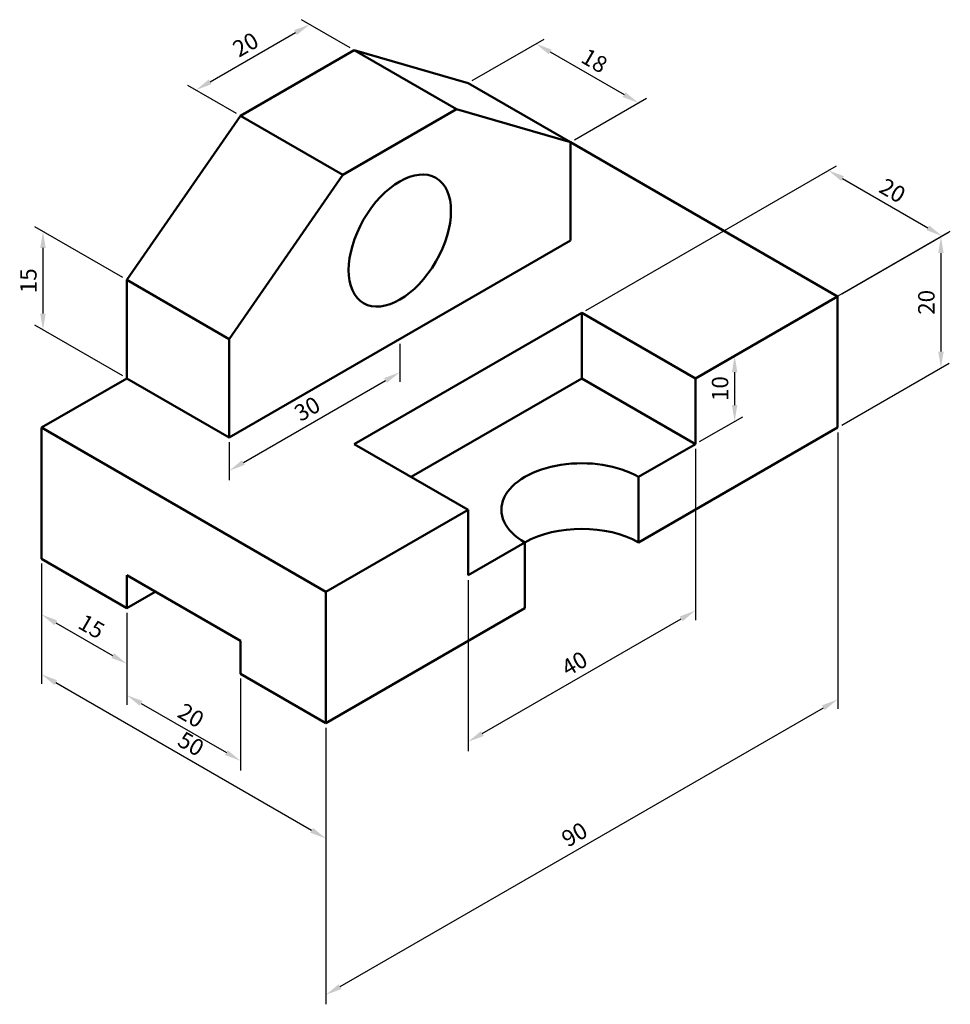
# Model space of a CAD drawing. Units: millimetres. Extents: x 3965 to 4107, y 1476 to 1626.
import ezdxf

# ---------------------------------------------------------------- set-up
doc = ezdxf.new("R2010")
doc.units = ezdxf.units.MM
doc.layers.add('M-DIMS', color=2, linetype='Continuous', lineweight=25)
doc.layers.add('M-OUTL', color=7, linetype='Continuous', lineweight=50)
doc.styles.get("Standard").update_dxf_attribs({"font": 'arial.ttf'})
doc.dimstyles.new('ISO-25', dxfattribs={"dimtxt": 2.5, "dimasz": 2.5, "dimexe": 1.25, "dimexo": 0.625, "dimtad": 1, "dimtxsty": 'Standard', "dimcen": 2.5, "dimadec": 0, "dimazin": 0, "dimtfac": 1, "dimtmove": 0, "dimatfit": 3, "dimfxl": 1, "dimarcsym": 0})

# ---------------------------------------------------------------- blocks, each defined once
blk = doc.blocks.new('*D1')
at = {"layer": 'Defpoints', "color": 0, "transparency": 16777216}
for p in [(3968.18, 1543.38), (4011.48, 1518.38), (4011.48, 1500.79)]:
    blk.add_point(p, dxfattribs=at)
at = {"layer": 'M-DIMS', "color": 0, "lineweight": -2, "transparency": 16777216}
for p, q in [((3968.18, 1542.66), (3968.18, 1524.34)), ((3970.35, 1524.54), (4009.32, 1502.04)), ((4011.48, 1517.66), (4011.48, 1499.34))]:
    blk.add_line(p, q, dxfattribs=at)
at = {"layer": 'M-DIMS', "color": 0, "transparency": 16777216}
for points in [[(3970.56, 1524.9), (3970.14, 1524.17), (3968.18, 1525.79)], [(4009.53, 1502.4), (4009.11, 1501.67), (4011.48, 1500.79)]]:
    blk.add_solid(points, dxfattribs=at)
at = {"layer": 'M-DIMS', "color": 0, "transparency": 16777216, "insert": (3990.78, 1514.93), "char_height": 2.5, "attachment_point": 5, "rotation": 330}
blk.add_mtext('50', dxfattribs=at)
blk = doc.blocks.new('*D2')
at = {"layer": 'Defpoints', "color": 0, "transparency": 16777216}
for p in [(3968.18, 1543.38), (3981.17, 1535.88), (3981.17, 1527.41)]:
    blk.add_point(p, dxfattribs=at)
at = {"layer": 'M-DIMS', "color": 0, "lineweight": -2, "transparency": 16777216}
for p, q in [((3968.18, 1542.66), (3968.18, 1533.47)), ((3981.17, 1535.16), (3981.17, 1525.97)), ((3970.35, 1533.66), (3979.01, 1528.66))]:
    blk.add_line(p, q, dxfattribs=at)
at = {"layer": 'M-DIMS', "color": 0, "transparency": 16777216}
for points in [[(3970.56, 1534.02), (3970.14, 1533.3), (3968.18, 1534.91)], [(3979.22, 1529.02), (3978.8, 1528.3), (3981.17, 1527.41)]]:
    blk.add_solid(points, dxfattribs=at)
at = {"layer": 'M-DIMS', "color": 0, "transparency": 16777216, "insert": (3975.63, 1532.81), "char_height": 2.5, "attachment_point": 5, "rotation": 330}
blk.add_mtext('15', dxfattribs=at)
blk = doc.blocks.new('*D3')
at = {"layer": 'Defpoints', "color": 0, "transparency": 16777216}
for p in [(3981.17, 1535.88), (3998.49, 1525.88), (3998.49, 1512.62)]:
    blk.add_point(p, dxfattribs=at)
at = {"layer": 'M-DIMS', "color": 0, "lineweight": -2, "transparency": 16777216}
for p, q in [((3981.17, 1535.16), (3981.17, 1521.17)), ((3998.49, 1525.16), (3998.49, 1511.17)), ((3983.34, 1521.37), (3996.33, 1513.87))]:
    blk.add_line(p, q, dxfattribs=at)
at = {"layer": 'M-DIMS', "color": 0, "transparency": 16777216}
for points in [[(3983.55, 1521.73), (3983.13, 1521.01), (3981.17, 1522.62)], [(3996.54, 1514.23), (3996.12, 1513.51), (3998.49, 1512.62)]]:
    blk.add_solid(points, dxfattribs=at)
at = {"layer": 'M-DIMS', "color": 0, "transparency": 16777216, "insert": (3990.78, 1519.26), "char_height": 2.5, "attachment_point": 5, "rotation": 330}
blk.add_mtext('20', dxfattribs=at)
blk = doc.blocks.new('*D4')
at = {"layer": 'Defpoints', "color": 0, "transparency": 16777216}
for p in [(4089.43, 1563.38), (4089.43, 1521.97), (4011.48, 1518.38)]:
    blk.add_point(p, dxfattribs=at)
at = {"layer": 'M-DIMS', "color": 0, "lineweight": -2, "transparency": 16777216}
for p, q in [((4089.43, 1562.66), (4089.43, 1520.53)), ((4013.65, 1478.22), (4087.26, 1520.72)), ((4011.48, 1517.66), (4011.48, 1475.53))]:
    blk.add_line(p, q, dxfattribs=at)
at = {"layer": 'M-DIMS', "color": 0, "transparency": 16777216}
for points in [[(4087.05, 1521.08), (4087.47, 1520.36), (4089.43, 1521.97)], [(4013.44, 1478.58), (4013.86, 1477.86), (4011.48, 1476.97)]]:
    blk.add_solid(points, dxfattribs=at)
at = {"layer": 'M-DIMS', "color": 0, "transparency": 16777216, "insert": (4049.5, 1501.12), "char_height": 2.5, "attachment_point": 5, "rotation": 30}
blk.add_mtext('90', dxfattribs=at)
blk = doc.blocks.new('*D5')
at = {"layer": 'Defpoints', "color": 0, "transparency": 16777216}
for p in [(4067.77, 1560.88), (4033.13, 1540.88), (4067.77, 1535.52)]:
    blk.add_point(p, dxfattribs=at)
at = {"layer": 'M-DIMS', "color": 0, "lineweight": -2, "transparency": 16777216}
for p, q in [((4067.77, 1560.16), (4067.77, 1534.07)), ((4033.13, 1540.16), (4033.13, 1514.07)), ((4035.3, 1516.77), (4065.61, 1534.27))]:
    blk.add_line(p, q, dxfattribs=at)
at = {"layer": 'M-DIMS', "color": 0, "transparency": 16777216}
for points in [[(4065.4, 1534.63), (4065.82, 1533.9), (4067.77, 1535.52)], [(4035.09, 1517.13), (4035.51, 1516.4), (4033.13, 1515.52)]]:
    blk.add_solid(points, dxfattribs=at)
at = {"layer": 'M-DIMS', "color": 0, "transparency": 16777216, "insert": (4049.5, 1527.16), "char_height": 2.5, "attachment_point": 5, "rotation": 30}
blk.add_mtext('40', dxfattribs=at)
blk = doc.blocks.new('*D6')
at = {"layer": 'Defpoints', "color": 0, "transparency": 16777216}
for p in [(4105.33, 1592.57), (4050.45, 1580.88), (4067.77, 1570.88)]:
    blk.add_point(p, dxfattribs=at)
at = {"layer": 'M-DIMS', "color": 0, "lineweight": -2, "transparency": 16777216}
for p, q in [((4051.08, 1581.25), (4089.26, 1603.29)), ((4090.18, 1601.32), (4103.17, 1593.82)), ((4068.4, 1571.25), (4106.58, 1593.29))]:
    blk.add_line(p, q, dxfattribs=at)
at = {"layer": 'M-DIMS', "color": 0, "transparency": 16777216}
for points in [[(4090.39, 1601.68), (4089.97, 1600.96), (4088.01, 1602.57)], [(4103.38, 1594.18), (4102.96, 1593.46), (4105.33, 1592.57)]]:
    blk.add_solid(points, dxfattribs=at)
at = {"layer": 'M-DIMS', "color": 0, "transparency": 16777216, "insert": (4097.62, 1599.22), "char_height": 2.5, "attachment_point": 5, "rotation": 330}
blk.add_mtext('20', dxfattribs=at)
blk = doc.blocks.new('*D7')
at = {"layer": 'Defpoints', "color": 0, "transparency": 16777216}
for p in [(4089.43, 1583.38), (4105.16, 1572.47), (4089.43, 1563.38)]:
    blk.add_point(p, dxfattribs=at)
at = {"layer": 'M-DIMS', "color": 0, "lineweight": -2, "transparency": 16777216}
for p, q in [((4090.05, 1583.75), (4106.41, 1593.19)), ((4105.16, 1589.97), (4105.16, 1574.97)), ((4090.05, 1563.75), (4106.41, 1573.19))]:
    blk.add_line(p, q, dxfattribs=at)
at = {"layer": 'M-DIMS', "color": 0, "transparency": 16777216}
for points in [[(4104.74, 1589.97), (4105.58, 1589.97), (4105.16, 1592.47)], [(4104.74, 1574.97), (4105.58, 1574.97), (4105.16, 1572.47)]]:
    blk.add_solid(points, dxfattribs=at)
at = {"layer": 'M-DIMS', "color": 0, "transparency": 16777216, "insert": (4103.26, 1582.47), "char_height": 2.5, "attachment_point": 5, "rotation": 90}
blk.add_mtext('20', dxfattribs=at)
blk = doc.blocks.new('*D8')
at = {"layer": 'Defpoints', "color": 0, "transparency": 16777216}
for p in [(4067.77, 1570.88), (4073.74, 1564.33), (4067.77, 1560.88)]:
    blk.add_point(p, dxfattribs=at)
at = {"layer": 'M-DIMS', "color": 0, "lineweight": -2, "transparency": 16777216}
for p, q in [((4068.4, 1571.25), (4074.99, 1575.05)), ((4073.74, 1571.83), (4073.74, 1566.83)), ((4068.4, 1561.25), (4074.99, 1565.05))]:
    blk.add_line(p, q, dxfattribs=at)
at = {"layer": 'M-DIMS', "color": 0, "transparency": 16777216}
for points in [[(4073.32, 1571.83), (4074.15, 1571.83), (4073.74, 1574.33)], [(4073.32, 1566.83), (4074.15, 1566.83), (4073.74, 1564.33)]]:
    blk.add_solid(points, dxfattribs=at)
at = {"layer": 'M-DIMS', "color": 0, "transparency": 16777216, "insert": (4071.84, 1569.33), "char_height": 2.5, "attachment_point": 5, "rotation": 90}
blk.add_mtext('10', dxfattribs=at)
blk = doc.blocks.new('*D9')
at = {"layer": 'Defpoints', "color": 0, "transparency": 16777216}
for p in [(4033.13, 1615.88), (4059.07, 1612.86), (4048.72, 1606.88)]:
    blk.add_point(p, dxfattribs=at)
at = {"layer": 'M-DIMS', "color": 0, "lineweight": -2, "transparency": 16777216}
for p, q in [((4033.76, 1616.25), (4044.73, 1622.58)), ((4045.65, 1620.61), (4056.91, 1614.11)), ((4049.35, 1607.25), (4060.32, 1613.58))]:
    blk.add_line(p, q, dxfattribs=at)
at = {"layer": 'M-DIMS', "color": 0, "transparency": 16777216}
for points in [[(4045.86, 1620.97), (4045.44, 1620.25), (4043.48, 1621.86)], [(4057.12, 1614.47), (4056.7, 1613.75), (4059.07, 1612.86)]]:
    blk.add_solid(points, dxfattribs=at)
at = {"layer": 'M-DIMS', "color": 0, "transparency": 16777216, "insert": (4052.23, 1619.01), "char_height": 2.5, "attachment_point": 5, "rotation": 330}
blk.add_mtext('18', dxfattribs=at)
blk = doc.blocks.new('*D10')
at = {"layer": 'Defpoints', "color": 0, "transparency": 16777216}
for p in [(4009.02, 1624.81), (4015.81, 1620.88), (3998.49, 1610.88)]:
    blk.add_point(p, dxfattribs=at)
at = {"layer": 'M-DIMS', "color": 0, "lineweight": -2, "transparency": 16777216}
for p, q in [((4015.19, 1621.25), (4007.77, 1625.53)), ((3993.86, 1616.06), (4006.85, 1623.56)), ((3997.87, 1611.25), (3990.45, 1615.53))]:
    blk.add_line(p, q, dxfattribs=at)
at = {"layer": 'M-DIMS', "color": 0, "transparency": 16777216}
for points in [[(4006.64, 1623.92), (4007.06, 1623.2), (4009.02, 1624.81)], [(3993.65, 1616.42), (3994.07, 1615.7), (3991.7, 1614.81)]]:
    blk.add_solid(points, dxfattribs=at)
at = {"layer": 'M-DIMS', "color": 0, "transparency": 16777216, "insert": (3999.41, 1621.46), "char_height": 2.5, "attachment_point": 5, "rotation": 30}
blk.add_mtext('20', dxfattribs=at)
blk = doc.blocks.new('*D11')
at = {"layer": 'Defpoints', "color": 0, "transparency": 16777216}
for p in [(3981.17, 1585.88), (3968.4, 1578.26), (3981.17, 1570.88)]:
    blk.add_point(p, dxfattribs=at)
at = {"layer": 'M-DIMS', "color": 0, "lineweight": -2, "transparency": 16777216}
for p, q in [((3980.55, 1586.25), (3967.15, 1593.98)), ((3968.4, 1590.76), (3968.4, 1580.76)), ((3980.55, 1571.25), (3967.15, 1578.98))]:
    blk.add_line(p, q, dxfattribs=at)
at = {"layer": 'M-DIMS', "color": 0, "transparency": 16777216}
for points in [[(3967.98, 1590.76), (3968.81, 1590.76), (3968.4, 1593.26)], [(3967.98, 1580.76), (3968.81, 1580.76), (3968.4, 1578.26)]]:
    blk.add_solid(points, dxfattribs=at)
at = {"layer": 'M-DIMS', "color": 0, "transparency": 16777216, "insert": (3966.5, 1585.76), "char_height": 2.5, "attachment_point": 5, "rotation": 90}
blk.add_mtext('15', dxfattribs=at)
blk = doc.blocks.new('*D12')
at = {"layer": 'Defpoints', "color": 0, "transparency": 16777216}
for p in [(4022.74, 1576.88), (4022.74, 1571.82), (3996.76, 1561.88)]:
    blk.add_point(p, dxfattribs=at)
at = {"layer": 'M-DIMS', "color": 0, "lineweight": -2, "transparency": 16777216}
for p, q in [((4022.74, 1576.16), (4022.74, 1570.38)), ((3998.93, 1558.07), (4020.58, 1570.57)), ((3996.76, 1561.16), (3996.76, 1555.38))]:
    blk.add_line(p, q, dxfattribs=at)
at = {"layer": 'M-DIMS', "color": 0, "transparency": 16777216}
for points in [[(4020.37, 1570.93), (4020.78, 1570.21), (4022.74, 1571.82)], [(3998.72, 1558.43), (3999.13, 1557.71), (3996.76, 1556.82)]]:
    blk.add_solid(points, dxfattribs=at)
at = {"layer": 'M-DIMS', "color": 0, "transparency": 16777216, "insert": (4008.8, 1565.97), "char_height": 2.5, "attachment_point": 5, "rotation": 30}
blk.add_mtext('30', dxfattribs=at)

msp = doc.modelspace()

# ---------------------------------------------------------------- linework, layer by layer
at = {"layer": 'M-OUTL'}
for p, q in [((3998.493, 1610.884), (4015.813, 1620.884)), ((4031.402, 1611.884), (4015.813, 1620.884)), ((4015.813, 1620.884), (4033.134, 1615.884)), ((4048.722, 1606.884), (4033.134, 1615.884)), ((4031.402, 1611.884), (4014.081, 1601.884)), ((4031.402, 1611.884), (4048.722, 1606.884)), ((3981.172, 1585.884), (3998.493, 1610.884)), ((4014.081, 1601.884), (3998.493, 1610.884)), ((4089.426, 1583.384), (4048.722, 1606.884)), ((4048.722, 1591.884), (4048.722, 1606.884)), ((4014.081, 1601.884), (3996.761, 1576.884)), ((3996.761, 1561.884), (4048.722, 1591.884)), ((3981.172, 1570.884), (3981.172, 1585.884)), ((3981.172, 1585.884), (3996.761, 1576.884)), ((4089.426, 1583.384), (4067.775, 1570.884)), ((4089.426, 1563.384), (4089.426, 1583.384)), ((4015.813, 1560.884), (4050.454, 1580.884)), ((4050.454, 1580.884), (4067.775, 1570.884)), ((4050.454, 1570.884), (4050.454, 1580.884)), ((3996.761, 1576.884), (3996.761, 1561.884)), ((3968.182, 1563.384), (3981.172, 1570.884)), ((3996.761, 1561.884), (3981.172, 1570.884)), ((4050.454, 1570.884), (4024.474, 1555.884)), ((4067.775, 1560.884), (4050.454, 1570.884)), ((4067.775, 1570.884), (4067.775, 1560.884)), ((3968.182, 1543.384), (3968.182, 1563.384)), ((3968.182, 1563.384), (4011.483, 1538.384)), ((4059.115, 1545.884), (4089.426, 1563.384)), ((4033.134, 1550.884), (4015.813, 1560.884)), ((4067.775, 1560.884), (4059.115, 1555.884)), ((4059.115, 1555.884), (4059.115, 1545.884)), ((4033.134, 1550.884), (4011.483, 1538.384)), ((4033.134, 1540.884), (4033.134, 1550.884)), ((4041.794, 1545.884), (4033.134, 1540.884)), ((4041.794, 1535.884), (4041.794, 1545.884)), ((3981.172, 1535.884), (3968.182, 1543.384)), ((3998.493, 1530.884), (3981.172, 1540.884)), ((3981.172, 1540.884), (3981.172, 1535.884)), ((3981.172, 1535.884), (3985.502, 1538.384)), ((4011.483, 1538.384), (4011.483, 1518.384)), ((4011.483, 1518.384), (4041.794, 1535.884)), ((4011.483, 1518.384), (4041.794, 1535.884)), ((3998.493, 1525.884), (3998.493, 1530.884)), ((4011.483, 1518.384), (3998.493, 1525.884))]:
    msp.add_line(p, q, dxfattribs=at)
msp.add_ellipse((4022.742, 1591.884), major_axis=(-5.511, -9.546), ratio=0.5773503, dxfattribs=at)
for centre, end_param in [((4050.454, 1550.884), 7.0685835), ((4050.454, 1540.884), 5.4977871)]:
    msp.add_ellipse(centre, major_axis=(-12.247, 0), ratio=0.5773503, start_param=3.9269908, end_param=end_param, dxfattribs=at)

# ---------------------------------------------------------------- dimensions: what is measured, and where the dimension line sits
at = {"layer": 'M-DIMS'}
for p1, p2, distance, picture, middle in [((3998.493, 1610.884), (4015.813, 1620.884), 6.797, '*D10', (3999.405, 1621.455)), ((4033.134, 1615.884), (4048.722, 1606.884), 10.35, '*D9', (4052.229, 1619.007)), ((4050.454, 1580.884), (4067.775, 1570.884), 37.558, '*D6', (4097.624, 1599.215)), ((3981.172, 1585.884), (3981.172, 1570.884), -12.776, '*D11', (3966.495, 1585.761)), ((4089.426, 1583.384), (4089.426, 1563.384), 15.736, '*D7', (4103.26, 1582.47)), ((3996.761, 1561.884), (4022.742, 1576.884), -4.387, '*D12', (4008.8, 1565.966)), ((4067.775, 1570.884), (4067.775, 1560.884), 5.963, '*D8', (4071.836, 1569.327)), ((4011.483, 1518.384), (4089.426, 1563.384), -35.864, '*D4', (4049.504, 1501.118)), ((4033.134, 1540.884), (4067.775, 1560.884), -21.97, '*D5', (4049.504, 1527.162)), ((3968.182, 1543.384), (4011.483, 1518.384), -15.241, '*D1', (3990.783, 1514.932)), ((3968.182, 1543.384), (3981.172, 1535.884), -7.34, '*D2', (3975.628, 1532.806)), ((3981.172, 1535.884), (3998.493, 1525.884), -11.491, '*D3', (3990.783, 1519.263))]:
    dim = msp.add_aligned_dim(p1=p1, p2=p2, distance=distance, dimstyle='ISO-25', override={"dimclrd": 0, "dimclre": 0, "dimclrt": 0}, dxfattribs=at)
    dim.commit()
    dim.dimension.update_dxf_attribs({"geometry": picture, "text_midpoint": middle})

doc.saveas('drawing.dxf')
